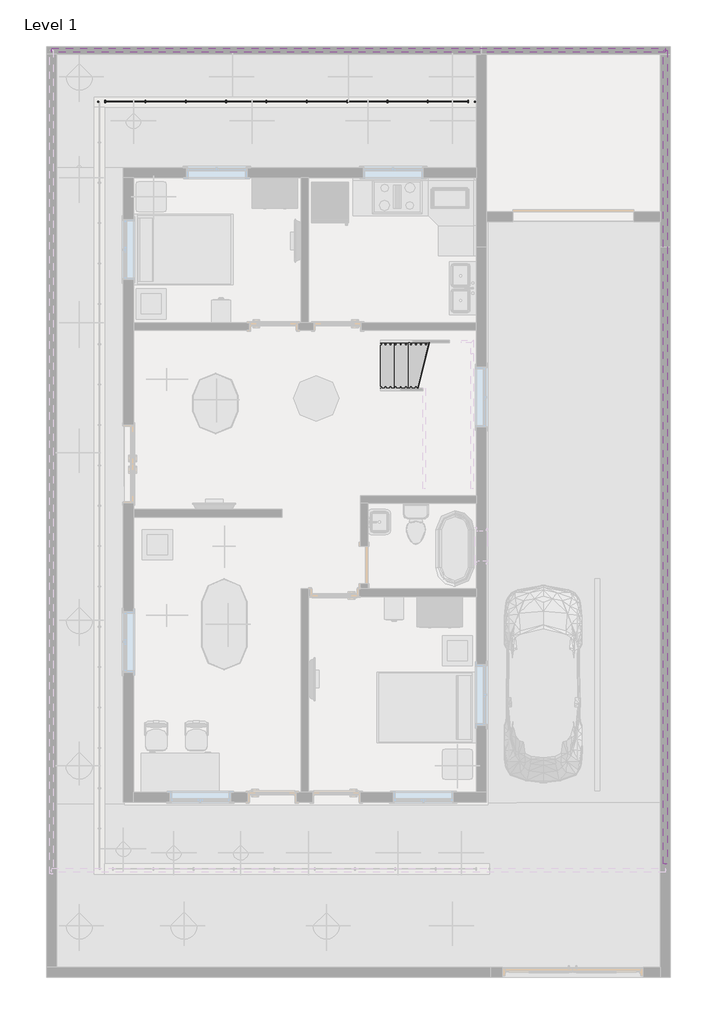
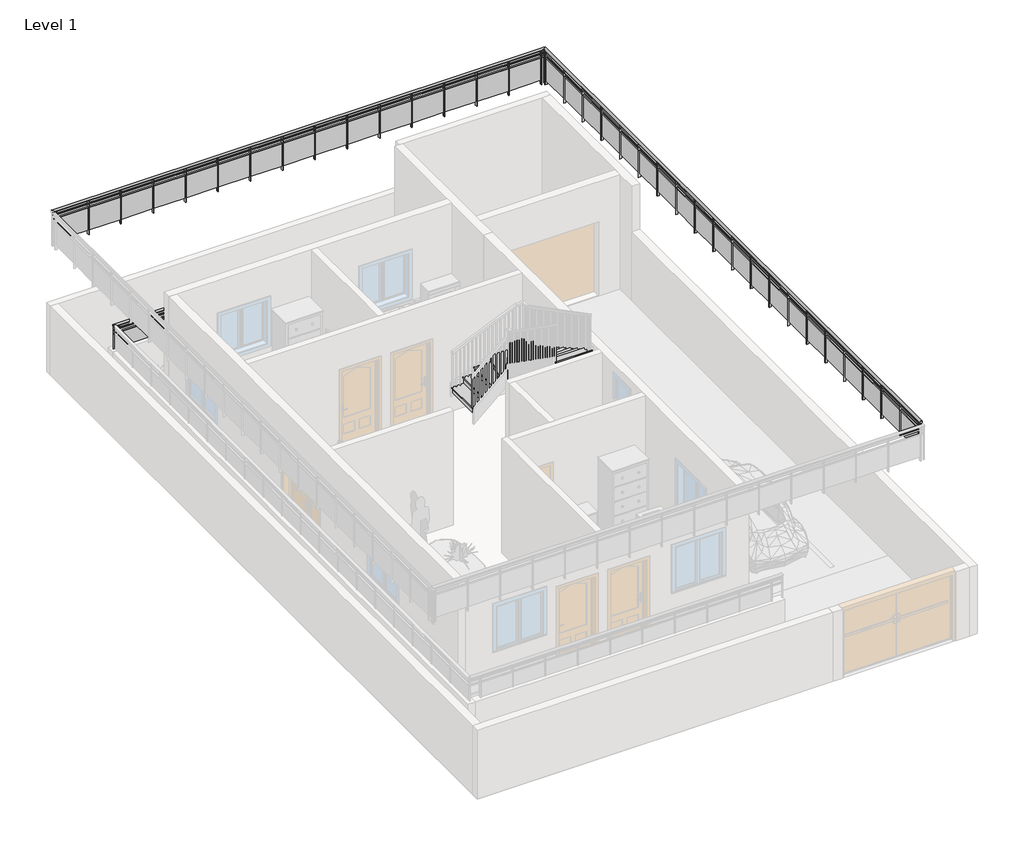
# One storey, part 4 of 5: 3 railings, 1 stair flight.
"""IFC4 building model written with IfcOpenShell, lengths in millimetres."""

from ifc_helpers import new_model, si_unit, point, frame, origin, place, context, project, spatial, polyline, ellipse_curve, trimmed, outline, extrude, transform, mapped, element, save
from ifc_brep_helpers import plane_surface, extruded_surface, advanced_brep
from components import stair_flight_29561c67

model = new_model("IFC4")

# Units and contexts
model_context = context("Model", 3, world=origin())
ifc_project = project(units=[si_unit("LENGTHUNIT", "METRE", prefix="MILLI")], contexts=[model_context])

# Site, building, storey
site = spatial("IfcSite", under=ifc_project)
building = spatial("IfcBuilding", under=site)
storey = spatial("IfcBuildingStorey", under=building, Name="Level 1", Elevation=0.0)

# Railings
placement = place(None, origin())
element("IfcRailing", 1, ObjectType="Glass Panel - Bottom Fill", at=placement, inside=storey, context=model_context, shape_type="SolidModel", body=[
    advanced_brep(
    [(-10096.3350785, 10613.9533005, 1524.0), (-10096.3350785, 10537.7533005, 1524.0), (-2501.7350785, 10613.9533005, 1524.0), (-2501.7350785, 10537.7533005, 1524.0)],
    [
        (0, 1, ellipse_curve(frame((-10096.3350785, 10575.8533005, 1524.0), z_axis=(-1.0, 0.0, 0.0), x_axis=(0.0, -1.0, 0.0)), 38.1, 28.575)),
        (1, 0, ellipse_curve(frame((-10096.3350785, 10575.8533005, 1524.0), z_axis=(-1.0, 0.0, 0.0), x_axis=(0.0, -1.0, 0.0)), 38.1, 28.575)),
        (2, 3, ellipse_curve(frame((-2501.7350785, 10575.8533005, 1524.0), z_axis=(1.0, 0.0, 0.0), x_axis=(0.0, -1.0, 0.0)), 38.1, 28.575)),
        (3, 2, ellipse_curve(frame((-2501.7350785, 10575.8533005, 1524.0), z_axis=(1.0, 0.0, 0.0), x_axis=(0.0, -1.0, 0.0)), 38.1, 28.575)),
        (0, 2),
        (3, 1),
    ],
    [
        plane_surface(frame((-10096.3350785, 10575.8533005, 1524.0), z_axis=(-1.0, 0.0, 0.0), x_axis=(0.0, 1.0, 0.0))),
        plane_surface(frame((-2501.7350785, 10575.8533005, 1524.0), z_axis=(1.0, 0.0, 0.0), x_axis=(0.0, 1.0, 0.0))),
        extruded_surface(trimmed(ellipse_curve(frame((-2501.7350785, 10575.8533005, 1524.0), z_axis=(-1.0, 0.0, 0.0), x_axis=(0.0, -1.0, 0.0)), 38.1, 28.575), [point((-2501.7350785, 10613.9533005, 1524.0))], [point((-2501.7350785, 10537.7533005, 1524.0))], True, "CARTESIAN"), (-7594.6, 0.0, 0.0), 7594.6),
        extruded_surface(trimmed(ellipse_curve(frame((-2501.7350785, 10575.8533005, 1524.0), z_axis=(-1.0, 0.0, 0.0), x_axis=(0.0, -1.0, 0.0)), 38.1, 28.575), [point((-2501.7350785, 10537.7533005, 1524.0))], [point((-2501.7350785, 10613.9533005, 1524.0))], True, "CARTESIAN"), (-7594.6, 0.0, 0.0), 7594.6),
    ],
    [
        (0, [[1, 2]]),
        (1, [[3, 4]]),
        (2, [[-1, 5, -4, 6]]),
        (3, [[-2, -6, -3, -5]]),
    ],
),
    extrude(outline(polyline([(-10096.3350785, 10563.1533005), (-10096.3350785, 10588.5533005), (-2501.7350785, 10588.5533005), (-2501.7350785, 10563.1533005), (-10096.3350785, 10563.1533005)])), frame((0.0, 0.0, 1409.7), z_axis=(0.0, 0.0, 1.0), x_axis=(1.0, 0.0, 0.0)), (0.0, 0.0, 1.0), 25.4),
    extrude(outline(polyline([(-10096.3350785, 10563.1533005), (-10096.3350785, 10588.5533005), (-2501.7350785, 10588.5533005), (-2501.7350785, 10563.1533005), (-10096.3350785, 10563.1533005)])), frame((0.0, 0.0, 1308.1), z_axis=(0.0, 0.0, 1.0), x_axis=(1.0, 0.0, 0.0)), (0.0, 0.0, 1.0), 25.4),
    extrude(outline(polyline([(-2647.7850785, 10550.4533005), (-2647.7850785, 10601.2533005), (-2635.0850785, 10601.2533005), (-2635.0850785, 10550.4533005), (-2647.7850785, 10550.4533005)])), frame((0.0, 0.0, 609.6), z_axis=(0.0, 0.0, 1.0), x_axis=(1.0, 0.0, 0.0)), (0.0, 0.0, 1.0), 885.6788223),
    extrude(outline(polyline([(-3454.2350785, 10582.3884575), (-2641.4350785, 10582.3884575), (-2641.4350785, 10576.0384575), (-3454.2350785, 10576.0384575), (-3454.2350785, 10582.3884575)])), frame((0.0, 0.0, 711.2), z_axis=(0.0, 0.0, 1.0), x_axis=(1.0, 0.0, 0.0)), (0.0, 0.0, 1.0), 596.9),
    extrude(outline(polyline([(-3460.5850785, 10550.4533005), (-3460.5850785, 10601.2533005), (-3447.8850785, 10601.2533005), (-3447.8850785, 10550.4533005), (-3460.5850785, 10550.4533005)])), frame((0.0, 0.0, 609.6), z_axis=(0.0, 0.0, 1.0), x_axis=(1.0, 0.0, 0.0)), (0.0, 0.0, 1.0), 885.6788223),
    extrude(outline(polyline([(-4267.0350785, 10582.3884575), (-3454.2350785, 10582.3884575), (-3454.2350785, 10576.0384575), (-4267.0350785, 10576.0384575), (-4267.0350785, 10582.3884575)])), frame((0.0, 0.0, 711.2), z_axis=(0.0, 0.0, 1.0), x_axis=(1.0, 0.0, 0.0)), (0.0, 0.0, 1.0), 596.9),
    extrude(outline(polyline([(-4273.3850785, 10550.4533005), (-4273.3850785, 10601.2533005), (-4260.6850785, 10601.2533005), (-4260.6850785, 10550.4533005), (-4273.3850785, 10550.4533005)])), frame((0.0, 0.0, 609.6), z_axis=(0.0, 0.0, 1.0), x_axis=(1.0, 0.0, 0.0)), (0.0, 0.0, 1.0), 885.6788223),
    extrude(outline(polyline([(-5079.8350785, 10582.3884575), (-4267.0350785, 10582.3884575), (-4267.0350785, 10576.0384575), (-5079.8350785, 10576.0384575), (-5079.8350785, 10582.3884575)])), frame((0.0, 0.0, 711.2), z_axis=(0.0, 0.0, 1.0), x_axis=(1.0, 0.0, 0.0)), (0.0, 0.0, 1.0), 596.9),
    extrude(outline(polyline([(-5086.1850785, 10550.4533005), (-5086.1850785, 10601.2533005), (-5073.4850785, 10601.2533005), (-5073.4850785, 10550.4533005), (-5086.1850785, 10550.4533005)])), frame((0.0, 0.0, 609.6), z_axis=(0.0, 0.0, 1.0), x_axis=(1.0, 0.0, 0.0)), (0.0, 0.0, 1.0), 885.6788223),
    extrude(outline(polyline([(-5892.6350785, 10582.3884575), (-5079.8350785, 10582.3884575), (-5079.8350785, 10576.0384575), (-5892.6350785, 10576.0384575), (-5892.6350785, 10582.3884575)])), frame((0.0, 0.0, 711.2), z_axis=(0.0, 0.0, 1.0), x_axis=(1.0, 0.0, 0.0)), (0.0, 0.0, 1.0), 596.9),
    extrude(outline(polyline([(-5898.9850785, 10550.4533005), (-5898.9850785, 10601.2533005), (-5886.2850785, 10601.2533005), (-5886.2850785, 10550.4533005), (-5898.9850785, 10550.4533005)])), frame((0.0, 0.0, 609.6), z_axis=(0.0, 0.0, 1.0), x_axis=(1.0, 0.0, 0.0)), (0.0, 0.0, 1.0), 885.6788223),
    extrude(outline(polyline([(-6705.4350785, 10582.3884575), (-5892.6350785, 10582.3884575), (-5892.6350785, 10576.0384575), (-6705.4350785, 10576.0384575), (-6705.4350785, 10582.3884575)])), frame((0.0, 0.0, 711.2), z_axis=(0.0, 0.0, 1.0), x_axis=(1.0, 0.0, 0.0)), (0.0, 0.0, 1.0), 596.9),
    extrude(outline(polyline([(-6711.7850785, 10550.4533005), (-6711.7850785, 10601.2533005), (-6699.0850785, 10601.2533005), (-6699.0850785, 10550.4533005), (-6711.7850785, 10550.4533005)])), frame((0.0, 0.0, 609.6), z_axis=(0.0, 0.0, 1.0), x_axis=(1.0, 0.0, 0.0)), (0.0, 0.0, 1.0), 885.6788223),
    extrude(outline(polyline([(-7518.2350785, 10582.3884575), (-6705.4350785, 10582.3884575), (-6705.4350785, 10576.0384575), (-7518.2350785, 10576.0384575), (-7518.2350785, 10582.3884575)])), frame((0.0, 0.0, 711.2), z_axis=(0.0, 0.0, 1.0), x_axis=(1.0, 0.0, 0.0)), (0.0, 0.0, 1.0), 596.9),
    extrude(outline(polyline([(-7524.5850785, 10550.4533005), (-7524.5850785, 10601.2533005), (-7511.8850785, 10601.2533005), (-7511.8850785, 10550.4533005), (-7524.5850785, 10550.4533005)])), frame((0.0, 0.0, 609.6), z_axis=(0.0, 0.0, 1.0), x_axis=(1.0, 0.0, 0.0)), (0.0, 0.0, 1.0), 885.6788223),
    extrude(outline(polyline([(-8331.0350785, 10582.3884575), (-7518.2350785, 10582.3884575), (-7518.2350785, 10576.0384575), (-8331.0350785, 10576.0384575), (-8331.0350785, 10582.3884575)])), frame((0.0, 0.0, 711.2), z_axis=(0.0, 0.0, 1.0), x_axis=(1.0, 0.0, 0.0)), (0.0, 0.0, 1.0), 596.9),
    extrude(outline(polyline([(-8337.3850785, 10550.4533005), (-8337.3850785, 10601.2533005), (-8324.6850785, 10601.2533005), (-8324.6850785, 10550.4533005), (-8337.3850785, 10550.4533005)])), frame((0.0, 0.0, 609.6), z_axis=(0.0, 0.0, 1.0), x_axis=(1.0, 0.0, 0.0)), (0.0, 0.0, 1.0), 885.6788223),
    extrude(outline(polyline([(-9143.8350785, 10582.3884575), (-8331.0350785, 10582.3884575), (-8331.0350785, 10576.0384575), (-9143.8350785, 10576.0384575), (-9143.8350785, 10582.3884575)])), frame((0.0, 0.0, 711.2), z_axis=(0.0, 0.0, 1.0), x_axis=(1.0, 0.0, 0.0)), (0.0, 0.0, 1.0), 596.9),
    extrude(outline(polyline([(-9150.1850785, 10550.4533005), (-9150.1850785, 10601.2533005), (-9137.4850785, 10601.2533005), (-9137.4850785, 10550.4533005), (-9150.1850785, 10550.4533005)])), frame((0.0, 0.0, 609.6), z_axis=(0.0, 0.0, 1.0), x_axis=(1.0, 0.0, 0.0)), (0.0, 0.0, 1.0), 885.6788223),
    extrude(outline(polyline([(-9956.6350785, 10582.3884575), (-9143.8350785, 10582.3884575), (-9143.8350785, 10576.0384575), (-9956.6350785, 10576.0384575), (-9956.6350785, 10582.3884575)])), frame((0.0, 0.0, 711.2), z_axis=(0.0, 0.0, 1.0), x_axis=(1.0, 0.0, 0.0)), (0.0, 0.0, 1.0), 596.9),
    extrude(outline(polyline([(-9962.9850785, 10550.4533005), (-9962.9850785, 10601.2533005), (-9950.2850785, 10601.2533005), (-9950.2850785, 10550.4533005), (-9962.9850785, 10550.4533005)])), frame((0.0, 0.0, 609.6), z_axis=(0.0, 0.0, 1.0), x_axis=(1.0, 0.0, 0.0)), (0.0, 0.0, 1.0), 885.6788223),
    extrude(outline(polyline([(-2514.4350785, 10566.3283005), (-2514.4350785, 10585.3783005), (-2495.3850785, 10585.3783005), (-2495.3850785, 10566.3283005), (-2514.4350785, 10566.3283005)])), frame((0.0, 0.0, 609.6), z_axis=(0.0, 0.0, 1.0), x_axis=(1.0, 0.0, 0.0)), (0.0, 0.0, 1.0), 885.6788223),
    extrude(outline(polyline([(-10102.6850785, 10566.3283005), (-10102.6850785, 10585.3783005), (-10083.6350785, 10585.3783005), (-10083.6350785, 10566.3283005), (-10102.6850785, 10566.3283005)])), frame((0.0, 0.0, 609.6), z_axis=(0.0, 0.0, 1.0), x_axis=(1.0, 0.0, 0.0)), (0.0, 0.0, 1.0), 885.6788223),
])
element("IfcRailing", 2, ObjectType="Glass Panel - Bottom Fill", at=placement, inside=storey, context=model_context, shape_type="SolidModel", body=[
    advanced_brep(
    [(-11036.1350785, 11649.0033005, 4267.2), (-11036.1350785, 11572.8033005, 4267.2), (1333.6649215, 11649.0033005, 4267.2), (1333.6649215, 11572.8033005, 4267.2)],
    [
        (0, 1, ellipse_curve(frame((-11036.1350785, 11610.9033005, 4267.2), z_axis=(-1.0, 0.0, 0.0), x_axis=(0.0, -1.0, 0.0)), 38.1, 28.575)),
        (1, 0, ellipse_curve(frame((-11036.1350785, 11610.9033005, 4267.2), z_axis=(-1.0, 0.0, 0.0), x_axis=(0.0, -1.0, 0.0)), 38.1, 28.575)),
        (2, 3, ellipse_curve(frame((1333.6649215, 11610.9033005, 4267.2), z_axis=(1.0, 0.0, 0.0), x_axis=(0.0, -1.0, 0.0)), 38.1, 28.575)),
        (3, 2, ellipse_curve(frame((1333.6649215, 11610.9033005, 4267.2), z_axis=(1.0, 0.0, 0.0), x_axis=(0.0, -1.0, 0.0)), 38.1, 28.575)),
        (0, 2),
        (3, 1),
    ],
    [
        plane_surface(frame((-11036.1350785, 11610.9033005, 4267.2), z_axis=(-1.0, 0.0, 0.0), x_axis=(0.0, 1.0, 0.0))),
        plane_surface(frame((1333.6649215, 11610.9033005, 4267.2), z_axis=(1.0, 0.0, 0.0), x_axis=(0.0, 1.0, 0.0))),
        extruded_surface(trimmed(ellipse_curve(frame((1333.6649215, 11610.9033005, 4267.2), z_axis=(-1.0, 0.0, 0.0), x_axis=(0.0, -1.0, 0.0)), 38.1, 28.575), [point((1333.6649215, 11649.0033005, 4267.2))], [point((1333.6649215, 11572.8033005, 4267.2))], True, "CARTESIAN"), (-12369.8, 0.0, 0.0), 12369.8),
        extruded_surface(trimmed(ellipse_curve(frame((1333.6649215, 11610.9033005, 4267.2), z_axis=(-1.0, 0.0, 0.0), x_axis=(0.0, -1.0, 0.0)), 38.1, 28.575), [point((1333.6649215, 11572.8033005, 4267.2))], [point((1333.6649215, 11649.0033005, 4267.2))], True, "CARTESIAN"), (-12369.8, 0.0, 0.0), 12369.8),
    ],
    [
        (0, [[1, 2]]),
        (1, [[3, 4]]),
        (2, [[-1, 5, -4, 6]]),
        (3, [[-2, -6, -3, -5]]),
    ],
),
    extrude(outline(polyline([(-11036.1350785, 11598.2033005), (-11036.1350785, 11623.6033005), (1333.6649215, 11623.6033005), (1333.6649215, 11598.2033005), (-11036.1350785, 11598.2033005)])), frame((0.0, 0.0, 4152.9), z_axis=(0.0, 0.0, 1.0), x_axis=(1.0, 0.0, 0.0)), (0.0, 0.0, 1.0), 25.4),
    extrude(outline(polyline([(-11036.1350785, 11598.2033005), (-11036.1350785, 11623.6033005), (1333.6649215, 11623.6033005), (1333.6649215, 11598.2033005), (-11036.1350785, 11598.2033005)])), frame((0.0, 0.0, 4051.3), z_axis=(0.0, 0.0, 1.0), x_axis=(1.0, 0.0, 0.0)), (0.0, 0.0, 1.0), 25.4),
    extrude(outline(polyline([(1238.4149215, 11585.5033005), (1238.4149215, 11636.3033005), (1251.1149215, 11636.3033005), (1251.1149215, 11585.5033005), (1238.4149215, 11585.5033005)])), frame((0.0, 0.0, 3352.8), z_axis=(0.0, 0.0, 1.0), x_axis=(1.0, 0.0, 0.0)), (0.0, 0.0, 1.0), 885.6788223),
    extrude(outline(polyline([(431.9649215, 11617.4384575), (1244.7649215, 11617.4384575), (1244.7649215, 11611.0884575), (431.9649215, 11611.0884575), (431.9649215, 11617.4384575)])), frame((0.0, 0.0, 3454.4), z_axis=(0.0, 0.0, 1.0), x_axis=(1.0, 0.0, 0.0)), (0.0, 0.0, 1.0), 596.9),
    extrude(outline(polyline([(425.6149215, 11585.5033005), (425.6149215, 11636.3033005), (438.3149215, 11636.3033005), (438.3149215, 11585.5033005), (425.6149215, 11585.5033005)])), frame((0.0, 0.0, 3352.8), z_axis=(0.0, 0.0, 1.0), x_axis=(1.0, 0.0, 0.0)), (0.0, 0.0, 1.0), 885.6788223),
    extrude(outline(polyline([(-380.8350785, 11617.4384575), (431.9649215, 11617.4384575), (431.9649215, 11611.0884575), (-380.8350785, 11611.0884575), (-380.8350785, 11617.4384575)])), frame((0.0, 0.0, 3454.4), z_axis=(0.0, 0.0, 1.0), x_axis=(1.0, 0.0, 0.0)), (0.0, 0.0, 1.0), 596.9),
    extrude(outline(polyline([(-387.1850785, 11585.5033005), (-387.1850785, 11636.3033005), (-374.4850785, 11636.3033005), (-374.4850785, 11585.5033005), (-387.1850785, 11585.5033005)])), frame((0.0, 0.0, 3352.8), z_axis=(0.0, 0.0, 1.0), x_axis=(1.0, 0.0, 0.0)), (0.0, 0.0, 1.0), 885.6788223),
    extrude(outline(polyline([(-1193.6350785, 11617.4384575), (-380.8350785, 11617.4384575), (-380.8350785, 11611.0884575), (-1193.6350785, 11611.0884575), (-1193.6350785, 11617.4384575)])), frame((0.0, 0.0, 3454.4), z_axis=(0.0, 0.0, 1.0), x_axis=(1.0, 0.0, 0.0)), (0.0, 0.0, 1.0), 596.9),
    extrude(outline(polyline([(-1199.9850785, 11585.5033005), (-1199.9850785, 11636.3033005), (-1187.2850785, 11636.3033005), (-1187.2850785, 11585.5033005), (-1199.9850785, 11585.5033005)])), frame((0.0, 0.0, 3352.8), z_axis=(0.0, 0.0, 1.0), x_axis=(1.0, 0.0, 0.0)), (0.0, 0.0, 1.0), 885.6788223),
    extrude(outline(polyline([(-2006.4350785, 11617.4384575), (-1193.6350785, 11617.4384575), (-1193.6350785, 11611.0884575), (-2006.4350785, 11611.0884575), (-2006.4350785, 11617.4384575)])), frame((0.0, 0.0, 3454.4), z_axis=(0.0, 0.0, 1.0), x_axis=(1.0, 0.0, 0.0)), (0.0, 0.0, 1.0), 596.9),
    extrude(outline(polyline([(-2012.7850785, 11585.5033005), (-2012.7850785, 11636.3033005), (-2000.0850785, 11636.3033005), (-2000.0850785, 11585.5033005), (-2012.7850785, 11585.5033005)])), frame((0.0, 0.0, 3352.8), z_axis=(0.0, 0.0, 1.0), x_axis=(1.0, 0.0, 0.0)), (0.0, 0.0, 1.0), 885.6788223),
    extrude(outline(polyline([(-2819.2350785, 11617.4384575), (-2006.4350785, 11617.4384575), (-2006.4350785, 11611.0884575), (-2819.2350785, 11611.0884575), (-2819.2350785, 11617.4384575)])), frame((0.0, 0.0, 3454.4), z_axis=(0.0, 0.0, 1.0), x_axis=(1.0, 0.0, 0.0)), (0.0, 0.0, 1.0), 596.9),
    extrude(outline(polyline([(-2825.5850785, 11585.5033005), (-2825.5850785, 11636.3033005), (-2812.8850785, 11636.3033005), (-2812.8850785, 11585.5033005), (-2825.5850785, 11585.5033005)])), frame((0.0, 0.0, 3352.8), z_axis=(0.0, 0.0, 1.0), x_axis=(1.0, 0.0, 0.0)), (0.0, 0.0, 1.0), 885.6788223),
    extrude(outline(polyline([(-3632.0350785, 11617.4384575), (-2819.2350785, 11617.4384575), (-2819.2350785, 11611.0884575), (-3632.0350785, 11611.0884575), (-3632.0350785, 11617.4384575)])), frame((0.0, 0.0, 3454.4), z_axis=(0.0, 0.0, 1.0), x_axis=(1.0, 0.0, 0.0)), (0.0, 0.0, 1.0), 596.9),
    extrude(outline(polyline([(-3638.3850785, 11585.5033005), (-3638.3850785, 11636.3033005), (-3625.6850785, 11636.3033005), (-3625.6850785, 11585.5033005), (-3638.3850785, 11585.5033005)])), frame((0.0, 0.0, 3352.8), z_axis=(0.0, 0.0, 1.0), x_axis=(1.0, 0.0, 0.0)), (0.0, 0.0, 1.0), 885.6788223),
    extrude(outline(polyline([(-4444.8350785, 11617.4384575), (-3632.0350785, 11617.4384575), (-3632.0350785, 11611.0884575), (-4444.8350785, 11611.0884575), (-4444.8350785, 11617.4384575)])), frame((0.0, 0.0, 3454.4), z_axis=(0.0, 0.0, 1.0), x_axis=(1.0, 0.0, 0.0)), (0.0, 0.0, 1.0), 596.9),
    extrude(outline(polyline([(-4451.1850785, 11585.5033005), (-4451.1850785, 11636.3033005), (-4438.4850785, 11636.3033005), (-4438.4850785, 11585.5033005), (-4451.1850785, 11585.5033005)])), frame((0.0, 0.0, 3352.8), z_axis=(0.0, 0.0, 1.0), x_axis=(1.0, 0.0, 0.0)), (0.0, 0.0, 1.0), 885.6788223),
    extrude(outline(polyline([(-5257.6350785, 11617.4384575), (-4444.8350785, 11617.4384575), (-4444.8350785, 11611.0884575), (-5257.6350785, 11611.0884575), (-5257.6350785, 11617.4384575)])), frame((0.0, 0.0, 3454.4), z_axis=(0.0, 0.0, 1.0), x_axis=(1.0, 0.0, 0.0)), (0.0, 0.0, 1.0), 596.9),
    extrude(outline(polyline([(-5263.9850785, 11585.5033005), (-5263.9850785, 11636.3033005), (-5251.2850785, 11636.3033005), (-5251.2850785, 11585.5033005), (-5263.9850785, 11585.5033005)])), frame((0.0, 0.0, 3352.8), z_axis=(0.0, 0.0, 1.0), x_axis=(1.0, 0.0, 0.0)), (0.0, 0.0, 1.0), 885.6788223),
    extrude(outline(polyline([(-6070.4350785, 11617.4384575), (-5257.6350785, 11617.4384575), (-5257.6350785, 11611.0884575), (-6070.4350785, 11611.0884575), (-6070.4350785, 11617.4384575)])), frame((0.0, 0.0, 3454.4), z_axis=(0.0, 0.0, 1.0), x_axis=(1.0, 0.0, 0.0)), (0.0, 0.0, 1.0), 596.9),
    extrude(outline(polyline([(-6076.7850785, 11585.5033005), (-6076.7850785, 11636.3033005), (-6064.0850785, 11636.3033005), (-6064.0850785, 11585.5033005), (-6076.7850785, 11585.5033005)])), frame((0.0, 0.0, 3352.8), z_axis=(0.0, 0.0, 1.0), x_axis=(1.0, 0.0, 0.0)), (0.0, 0.0, 1.0), 885.6788223),
    extrude(outline(polyline([(-6883.2350785, 11617.4384575), (-6070.4350785, 11617.4384575), (-6070.4350785, 11611.0884575), (-6883.2350785, 11611.0884575), (-6883.2350785, 11617.4384575)])), frame((0.0, 0.0, 3454.4), z_axis=(0.0, 0.0, 1.0), x_axis=(1.0, 0.0, 0.0)), (0.0, 0.0, 1.0), 596.9),
    extrude(outline(polyline([(-6889.5850785, 11585.5033005), (-6889.5850785, 11636.3033005), (-6876.8850785, 11636.3033005), (-6876.8850785, 11585.5033005), (-6889.5850785, 11585.5033005)])), frame((0.0, 0.0, 3352.8), z_axis=(0.0, 0.0, 1.0), x_axis=(1.0, 0.0, 0.0)), (0.0, 0.0, 1.0), 885.6788223),
    extrude(outline(polyline([(-7696.0350785, 11617.4384575), (-6883.2350785, 11617.4384575), (-6883.2350785, 11611.0884575), (-7696.0350785, 11611.0884575), (-7696.0350785, 11617.4384575)])), frame((0.0, 0.0, 3454.4), z_axis=(0.0, 0.0, 1.0), x_axis=(1.0, 0.0, 0.0)), (0.0, 0.0, 1.0), 596.9),
    extrude(outline(polyline([(-7702.3850785, 11585.5033005), (-7702.3850785, 11636.3033005), (-7689.6850785, 11636.3033005), (-7689.6850785, 11585.5033005), (-7702.3850785, 11585.5033005)])), frame((0.0, 0.0, 3352.8), z_axis=(0.0, 0.0, 1.0), x_axis=(1.0, 0.0, 0.0)), (0.0, 0.0, 1.0), 885.6788223),
    extrude(outline(polyline([(-8508.8350785, 11617.4384575), (-7696.0350785, 11617.4384575), (-7696.0350785, 11611.0884575), (-8508.8350785, 11611.0884575), (-8508.8350785, 11617.4384575)])), frame((0.0, 0.0, 3454.4), z_axis=(0.0, 0.0, 1.0), x_axis=(1.0, 0.0, 0.0)), (0.0, 0.0, 1.0), 596.9),
    extrude(outline(polyline([(-8515.1850785, 11585.5033005), (-8515.1850785, 11636.3033005), (-8502.4850785, 11636.3033005), (-8502.4850785, 11585.5033005), (-8515.1850785, 11585.5033005)])), frame((0.0, 0.0, 3352.8), z_axis=(0.0, 0.0, 1.0), x_axis=(1.0, 0.0, 0.0)), (0.0, 0.0, 1.0), 885.6788223),
    extrude(outline(polyline([(-9321.6350785, 11617.4384575), (-8508.8350785, 11617.4384575), (-8508.8350785, 11611.0884575), (-9321.6350785, 11611.0884575), (-9321.6350785, 11617.4384575)])), frame((0.0, 0.0, 3454.4), z_axis=(0.0, 0.0, 1.0), x_axis=(1.0, 0.0, 0.0)), (0.0, 0.0, 1.0), 596.9),
    extrude(outline(polyline([(-9327.9850785, 11585.5033005), (-9327.9850785, 11636.3033005), (-9315.2850785, 11636.3033005), (-9315.2850785, 11585.5033005), (-9327.9850785, 11585.5033005)])), frame((0.0, 0.0, 3352.8), z_axis=(0.0, 0.0, 1.0), x_axis=(1.0, 0.0, 0.0)), (0.0, 0.0, 1.0), 885.6788223),
    extrude(outline(polyline([(-10134.4350785, 11617.4384575), (-9321.6350785, 11617.4384575), (-9321.6350785, 11611.0884575), (-10134.4350785, 11611.0884575), (-10134.4350785, 11617.4384575)])), frame((0.0, 0.0, 3454.4), z_axis=(0.0, 0.0, 1.0), x_axis=(1.0, 0.0, 0.0)), (0.0, 0.0, 1.0), 596.9),
    extrude(outline(polyline([(-10140.7850785, 11585.5033005), (-10140.7850785, 11636.3033005), (-10128.0850785, 11636.3033005), (-10128.0850785, 11585.5033005), (-10140.7850785, 11585.5033005)])), frame((0.0, 0.0, 3352.8), z_axis=(0.0, 0.0, 1.0), x_axis=(1.0, 0.0, 0.0)), (0.0, 0.0, 1.0), 885.6788223),
    extrude(outline(polyline([(-10947.2350785, 11617.4384575), (-10134.4350785, 11617.4384575), (-10134.4350785, 11611.0884575), (-10947.2350785, 11611.0884575), (-10947.2350785, 11617.4384575)])), frame((0.0, 0.0, 3454.4), z_axis=(0.0, 0.0, 1.0), x_axis=(1.0, 0.0, 0.0)), (0.0, 0.0, 1.0), 596.9),
    extrude(outline(polyline([(-10953.5850785, 11585.5033005), (-10953.5850785, 11636.3033005), (-10940.8850785, 11636.3033005), (-10940.8850785, 11585.5033005), (-10953.5850785, 11585.5033005)])), frame((0.0, 0.0, 3352.8), z_axis=(0.0, 0.0, 1.0), x_axis=(1.0, 0.0, 0.0)), (0.0, 0.0, 1.0), 885.6788223),
    extrude(outline(polyline([(1320.9649215, 11601.3783005), (1320.9649215, 11620.4283005), (1340.0149215, 11620.4283005), (1340.0149215, 11601.3783005), (1320.9649215, 11601.3783005)])), frame((0.0, 0.0, 3352.8), z_axis=(0.0, 0.0, 1.0), x_axis=(1.0, 0.0, 0.0)), (0.0, 0.0, 1.0), 885.6788223),
    extrude(outline(polyline([(-11042.4850785, 11601.3783005), (-11042.4850785, 11620.4283005), (-11023.4350785, 11620.4283005), (-11023.4350785, 11601.3783005), (-11042.4850785, 11601.3783005)])), frame((0.0, 0.0, 3352.8), z_axis=(0.0, 0.0, 1.0), x_axis=(1.0, 0.0, 0.0)), (0.0, 0.0, 1.0), 885.6788223),
])
element("IfcRailing", 3, ObjectType="Glass Panel - Bottom Fill", at=placement, inside=storey, context=model_context, shape_type="SolidModel", body=[
    advanced_brep(
    [(1371.7649215, 11610.9033005, 4267.2), (1295.5649215, 11610.9033005, 4267.2), (1371.7649215, -4772.0966995, 4267.2), (1295.5649215, -4772.0966995, 4267.2)],
    [
        (0, 1, ellipse_curve(frame((1333.6649215, 11610.9033005, 4267.2), z_axis=(0.0, 1.0, 0.0), x_axis=(-1.0, 0.0, 0.0)), 38.1, 28.575)),
        (1, 0, ellipse_curve(frame((1333.6649215, 11610.9033005, 4267.2), z_axis=(0.0, 1.0, 0.0), x_axis=(-1.0, 0.0, 0.0)), 38.1, 28.575)),
        (2, 3, ellipse_curve(frame((1333.6649215, -4772.0966995, 4267.2), z_axis=(0.0, -1.0, 0.0), x_axis=(-1.0, 0.0, 0.0)), 38.1, 28.575)),
        (3, 2, ellipse_curve(frame((1333.6649215, -4772.0966995, 4267.2), z_axis=(0.0, -1.0, 0.0), x_axis=(-1.0, 0.0, 0.0)), 38.1, 28.575)),
        (0, 2),
        (3, 1),
    ],
    [
        plane_surface(frame((1333.6649215, 11610.9033005, 4267.2), z_axis=(0.0, 1.0, 0.0), x_axis=(0.0, 0.0, -1.0))),
        plane_surface(frame((1333.6649215, -4772.0966995, 4267.2), z_axis=(0.0, -1.0, 0.0), x_axis=(0.0, 0.0, -1.0))),
        extruded_surface(trimmed(ellipse_curve(frame((1333.6649215, -4772.0966995, 4267.2), z_axis=(0.0, 1.0, 0.0), x_axis=(-1.0, 0.0, 0.0)), 38.1, 28.575), [point((1371.7649215, -4772.0966995, 4267.2))], [point((1295.5649215, -4772.0966995, 4267.2))], True, "CARTESIAN"), (0.0, 16383.0, 0.0), 16383.0),
        extruded_surface(trimmed(ellipse_curve(frame((1333.6649215, -4772.0966995, 4267.2), z_axis=(0.0, 1.0, 0.0), x_axis=(-1.0, 0.0, 0.0)), 38.1, 28.575), [point((1295.5649215, -4772.0966995, 4267.2))], [point((1371.7649215, -4772.0966995, 4267.2))], True, "CARTESIAN"), (0.0, 16383.0, 0.0), 16383.0),
    ],
    [
        (0, [[1, 2]]),
        (1, [[3, 4]]),
        (2, [[-1, 5, -4, 6]]),
        (3, [[-2, -6, -3, -5]]),
    ],
),
    extrude(outline(polyline([(1320.9649215, 11610.9033005), (1346.3649215, 11610.9033005), (1346.3649215, -4772.0966995), (1320.9649215, -4772.0966995), (1320.9649215, 11610.9033005)])), frame((0.0, 0.0, 4152.9), z_axis=(0.0, 0.0, 1.0), x_axis=(1.0, 0.0, 0.0)), (0.0, 0.0, 1.0), 25.4),
    extrude(outline(polyline([(1320.9649215, 11610.9033005), (1346.3649215, 11610.9033005), (1346.3649215, -4772.0966995), (1320.9649215, -4772.0966995), (1320.9649215, 11610.9033005)])), frame((0.0, 0.0, 4051.3), z_axis=(0.0, 0.0, 1.0), x_axis=(1.0, 0.0, 0.0)), (0.0, 0.0, 1.0), 25.4),
    extrude(outline(polyline([(1308.2649215, -4702.2466995), (1359.0649215, -4702.2466995), (1359.0649215, -4714.9466995), (1308.2649215, -4714.9466995), (1308.2649215, -4702.2466995)])), frame((0.0, 0.0, 3352.8), z_axis=(0.0, 0.0, 1.0), x_axis=(1.0, 0.0, 0.0)), (0.0, 0.0, 1.0), 885.6788223),
    extrude(outline(polyline([(1340.2000785, -3895.7966995), (1340.2000785, -4708.5966995), (1333.8500785, -4708.5966995), (1333.8500785, -3895.7966995), (1340.2000785, -3895.7966995)])), frame((0.0, 0.0, 3454.4), z_axis=(0.0, 0.0, 1.0), x_axis=(1.0, 0.0, 0.0)), (0.0, 0.0, 1.0), 596.9),
    extrude(outline(polyline([(1308.2649215, -3889.4466995), (1359.0649215, -3889.4466995), (1359.0649215, -3902.1466995), (1308.2649215, -3902.1466995), (1308.2649215, -3889.4466995)])), frame((0.0, 0.0, 3352.8), z_axis=(0.0, 0.0, 1.0), x_axis=(1.0, 0.0, 0.0)), (0.0, 0.0, 1.0), 885.6788223),
    extrude(outline(polyline([(1340.2000785, -3082.9966995), (1340.2000785, -3895.7966995), (1333.8500785, -3895.7966995), (1333.8500785, -3082.9966995), (1340.2000785, -3082.9966995)])), frame((0.0, 0.0, 3454.4), z_axis=(0.0, 0.0, 1.0), x_axis=(1.0, 0.0, 0.0)), (0.0, 0.0, 1.0), 596.9),
    extrude(outline(polyline([(1308.2649215, -3076.6466995), (1359.0649215, -3076.6466995), (1359.0649215, -3089.3466995), (1308.2649215, -3089.3466995), (1308.2649215, -3076.6466995)])), frame((0.0, 0.0, 3352.8), z_axis=(0.0, 0.0, 1.0), x_axis=(1.0, 0.0, 0.0)), (0.0, 0.0, 1.0), 885.6788223),
    extrude(outline(polyline([(1340.2000785, -2270.1966995), (1340.2000785, -3082.9966995), (1333.8500785, -3082.9966995), (1333.8500785, -2270.1966995), (1340.2000785, -2270.1966995)])), frame((0.0, 0.0, 3454.4), z_axis=(0.0, 0.0, 1.0), x_axis=(1.0, 0.0, 0.0)), (0.0, 0.0, 1.0), 596.9),
    extrude(outline(polyline([(1308.2649215, -2263.8466995), (1359.0649215, -2263.8466995), (1359.0649215, -2276.5466995), (1308.2649215, -2276.5466995), (1308.2649215, -2263.8466995)])), frame((0.0, 0.0, 3352.8), z_axis=(0.0, 0.0, 1.0), x_axis=(1.0, 0.0, 0.0)), (0.0, 0.0, 1.0), 885.6788223),
    extrude(outline(polyline([(1340.2000785, -1457.3966995), (1340.2000785, -2270.1966995), (1333.8500785, -2270.1966995), (1333.8500785, -1457.3966995), (1340.2000785, -1457.3966995)])), frame((0.0, 0.0, 3454.4), z_axis=(0.0, 0.0, 1.0), x_axis=(1.0, 0.0, 0.0)), (0.0, 0.0, 1.0), 596.9),
    extrude(outline(polyline([(1308.2649215, -1451.0466995), (1359.0649215, -1451.0466995), (1359.0649215, -1463.7466995), (1308.2649215, -1463.7466995), (1308.2649215, -1451.0466995)])), frame((0.0, 0.0, 3352.8), z_axis=(0.0, 0.0, 1.0), x_axis=(1.0, 0.0, 0.0)), (0.0, 0.0, 1.0), 885.6788223),
    extrude(outline(polyline([(1340.2000785, -644.5966995), (1340.2000785, -1457.3966995), (1333.8500785, -1457.3966995), (1333.8500785, -644.5966995), (1340.2000785, -644.5966995)])), frame((0.0, 0.0, 3454.4), z_axis=(0.0, 0.0, 1.0), x_axis=(1.0, 0.0, 0.0)), (0.0, 0.0, 1.0), 596.9),
    extrude(outline(polyline([(1308.2649215, -638.2466995), (1359.0649215, -638.2466995), (1359.0649215, -650.9466995), (1308.2649215, -650.9466995), (1308.2649215, -638.2466995)])), frame((0.0, 0.0, 3352.8), z_axis=(0.0, 0.0, 1.0), x_axis=(1.0, 0.0, 0.0)), (0.0, 0.0, 1.0), 885.6788223),
    extrude(outline(polyline([(1340.2000785, 168.2033005), (1340.2000785, -644.5966995), (1333.8500785, -644.5966995), (1333.8500785, 168.2033005), (1340.2000785, 168.2033005)])), frame((0.0, 0.0, 3454.4), z_axis=(0.0, 0.0, 1.0), x_axis=(1.0, 0.0, 0.0)), (0.0, 0.0, 1.0), 596.9),
    extrude(outline(polyline([(1308.2649215, 174.5533005), (1359.0649215, 174.5533005), (1359.0649215, 161.8533005), (1308.2649215, 161.8533005), (1308.2649215, 174.5533005)])), frame((0.0, 0.0, 3352.8), z_axis=(0.0, 0.0, 1.0), x_axis=(1.0, 0.0, 0.0)), (0.0, 0.0, 1.0), 885.6788223),
    extrude(outline(polyline([(1340.2000785, 981.0033005), (1340.2000785, 168.2033005), (1333.8500785, 168.2033005), (1333.8500785, 981.0033005), (1340.2000785, 981.0033005)])), frame((0.0, 0.0, 3454.4), z_axis=(0.0, 0.0, 1.0), x_axis=(1.0, 0.0, 0.0)), (0.0, 0.0, 1.0), 596.9),
    extrude(outline(polyline([(1308.2649215, 987.3533005), (1359.0649215, 987.3533005), (1359.0649215, 974.6533005), (1308.2649215, 974.6533005), (1308.2649215, 987.3533005)])), frame((0.0, 0.0, 3352.8), z_axis=(0.0, 0.0, 1.0), x_axis=(1.0, 0.0, 0.0)), (0.0, 0.0, 1.0), 885.6788223),
    extrude(outline(polyline([(1340.2000785, 1793.8033005), (1340.2000785, 981.0033005), (1333.8500785, 981.0033005), (1333.8500785, 1793.8033005), (1340.2000785, 1793.8033005)])), frame((0.0, 0.0, 3454.4), z_axis=(0.0, 0.0, 1.0), x_axis=(1.0, 0.0, 0.0)), (0.0, 0.0, 1.0), 596.9),
    extrude(outline(polyline([(1308.2649215, 1800.1533005), (1359.0649215, 1800.1533005), (1359.0649215, 1787.4533005), (1308.2649215, 1787.4533005), (1308.2649215, 1800.1533005)])), frame((0.0, 0.0, 3352.8), z_axis=(0.0, 0.0, 1.0), x_axis=(1.0, 0.0, 0.0)), (0.0, 0.0, 1.0), 885.6788223),
    extrude(outline(polyline([(1340.2000785, 2606.6033005), (1340.2000785, 1793.8033005), (1333.8500785, 1793.8033005), (1333.8500785, 2606.6033005), (1340.2000785, 2606.6033005)])), frame((0.0, 0.0, 3454.4), z_axis=(0.0, 0.0, 1.0), x_axis=(1.0, 0.0, 0.0)), (0.0, 0.0, 1.0), 596.9),
    extrude(outline(polyline([(1308.2649215, 2612.9533005), (1359.0649215, 2612.9533005), (1359.0649215, 2600.2533005), (1308.2649215, 2600.2533005), (1308.2649215, 2612.9533005)])), frame((0.0, 0.0, 3352.8), z_axis=(0.0, 0.0, 1.0), x_axis=(1.0, 0.0, 0.0)), (0.0, 0.0, 1.0), 885.6788223),
    extrude(outline(polyline([(1340.2000785, 3419.4033005), (1340.2000785, 2606.6033005), (1333.8500785, 2606.6033005), (1333.8500785, 3419.4033005), (1340.2000785, 3419.4033005)])), frame((0.0, 0.0, 3454.4), z_axis=(0.0, 0.0, 1.0), x_axis=(1.0, 0.0, 0.0)), (0.0, 0.0, 1.0), 596.9),
    extrude(outline(polyline([(1308.2649215, 3425.7533005), (1359.0649215, 3425.7533005), (1359.0649215, 3413.0533005), (1308.2649215, 3413.0533005), (1308.2649215, 3425.7533005)])), frame((0.0, 0.0, 3352.8), z_axis=(0.0, 0.0, 1.0), x_axis=(1.0, 0.0, 0.0)), (0.0, 0.0, 1.0), 885.6788223),
    extrude(outline(polyline([(1340.2000785, 4232.2033005), (1340.2000785, 3419.4033005), (1333.8500785, 3419.4033005), (1333.8500785, 4232.2033005), (1340.2000785, 4232.2033005)])), frame((0.0, 0.0, 3454.4), z_axis=(0.0, 0.0, 1.0), x_axis=(1.0, 0.0, 0.0)), (0.0, 0.0, 1.0), 596.9),
    extrude(outline(polyline([(1308.2649215, 4238.5533005), (1359.0649215, 4238.5533005), (1359.0649215, 4225.8533005), (1308.2649215, 4225.8533005), (1308.2649215, 4238.5533005)])), frame((0.0, 0.0, 3352.8), z_axis=(0.0, 0.0, 1.0), x_axis=(1.0, 0.0, 0.0)), (0.0, 0.0, 1.0), 885.6788223),
    extrude(outline(polyline([(1340.2000785, 5045.0033005), (1340.2000785, 4232.2033005), (1333.8500785, 4232.2033005), (1333.8500785, 5045.0033005), (1340.2000785, 5045.0033005)])), frame((0.0, 0.0, 3454.4), z_axis=(0.0, 0.0, 1.0), x_axis=(1.0, 0.0, 0.0)), (0.0, 0.0, 1.0), 596.9),
    extrude(outline(polyline([(1308.2649215, 5051.3533005), (1359.0649215, 5051.3533005), (1359.0649215, 5038.6533005), (1308.2649215, 5038.6533005), (1308.2649215, 5051.3533005)])), frame((0.0, 0.0, 3352.8), z_axis=(0.0, 0.0, 1.0), x_axis=(1.0, 0.0, 0.0)), (0.0, 0.0, 1.0), 885.6788223),
    extrude(outline(polyline([(1340.2000785, 5857.8033005), (1340.2000785, 5045.0033005), (1333.8500785, 5045.0033005), (1333.8500785, 5857.8033005), (1340.2000785, 5857.8033005)])), frame((0.0, 0.0, 3454.4), z_axis=(0.0, 0.0, 1.0), x_axis=(1.0, 0.0, 0.0)), (0.0, 0.0, 1.0), 596.9),
    extrude(outline(polyline([(1308.2649215, 5864.1533005), (1359.0649215, 5864.1533005), (1359.0649215, 5851.4533005), (1308.2649215, 5851.4533005), (1308.2649215, 5864.1533005)])), frame((0.0, 0.0, 3352.8), z_axis=(0.0, 0.0, 1.0), x_axis=(1.0, 0.0, 0.0)), (0.0, 0.0, 1.0), 885.6788223),
    extrude(outline(polyline([(1340.2000785, 6670.6033005), (1340.2000785, 5857.8033005), (1333.8500785, 5857.8033005), (1333.8500785, 6670.6033005), (1340.2000785, 6670.6033005)])), frame((0.0, 0.0, 3454.4), z_axis=(0.0, 0.0, 1.0), x_axis=(1.0, 0.0, 0.0)), (0.0, 0.0, 1.0), 596.9),
    extrude(outline(polyline([(1308.2649215, 6676.9533005), (1359.0649215, 6676.9533005), (1359.0649215, 6664.2533005), (1308.2649215, 6664.2533005), (1308.2649215, 6676.9533005)])), frame((0.0, 0.0, 3352.8), z_axis=(0.0, 0.0, 1.0), x_axis=(1.0, 0.0, 0.0)), (0.0, 0.0, 1.0), 885.6788223),
    extrude(outline(polyline([(1340.2000785, 7483.4033005), (1340.2000785, 6670.6033005), (1333.8500785, 6670.6033005), (1333.8500785, 7483.4033005), (1340.2000785, 7483.4033005)])), frame((0.0, 0.0, 3454.4), z_axis=(0.0, 0.0, 1.0), x_axis=(1.0, 0.0, 0.0)), (0.0, 0.0, 1.0), 596.9),
    extrude(outline(polyline([(1308.2649215, 7489.7533005), (1359.0649215, 7489.7533005), (1359.0649215, 7477.0533005), (1308.2649215, 7477.0533005), (1308.2649215, 7489.7533005)])), frame((0.0, 0.0, 3352.8), z_axis=(0.0, 0.0, 1.0), x_axis=(1.0, 0.0, 0.0)), (0.0, 0.0, 1.0), 885.6788223),
    extrude(outline(polyline([(1340.2000785, 8296.2033005), (1340.2000785, 7483.4033005), (1333.8500785, 7483.4033005), (1333.8500785, 8296.2033005), (1340.2000785, 8296.2033005)])), frame((0.0, 0.0, 3454.4), z_axis=(0.0, 0.0, 1.0), x_axis=(1.0, 0.0, 0.0)), (0.0, 0.0, 1.0), 596.9),
    extrude(outline(polyline([(1308.2649215, 8302.5533005), (1359.0649215, 8302.5533005), (1359.0649215, 8289.8533005), (1308.2649215, 8289.8533005), (1308.2649215, 8302.5533005)])), frame((0.0, 0.0, 3352.8), z_axis=(0.0, 0.0, 1.0), x_axis=(1.0, 0.0, 0.0)), (0.0, 0.0, 1.0), 885.6788223),
    extrude(outline(polyline([(1340.2000785, 9109.0033005), (1340.2000785, 8296.2033005), (1333.8500785, 8296.2033005), (1333.8500785, 9109.0033005), (1340.2000785, 9109.0033005)])), frame((0.0, 0.0, 3454.4), z_axis=(0.0, 0.0, 1.0), x_axis=(1.0, 0.0, 0.0)), (0.0, 0.0, 1.0), 596.9),
    extrude(outline(polyline([(1308.2649215, 9115.3533005), (1359.0649215, 9115.3533005), (1359.0649215, 9102.6533005), (1308.2649215, 9102.6533005), (1308.2649215, 9115.3533005)])), frame((0.0, 0.0, 3352.8), z_axis=(0.0, 0.0, 1.0), x_axis=(1.0, 0.0, 0.0)), (0.0, 0.0, 1.0), 885.6788223),
    extrude(outline(polyline([(1340.2000785, 9921.8033005), (1340.2000785, 9109.0033005), (1333.8500785, 9109.0033005), (1333.8500785, 9921.8033005), (1340.2000785, 9921.8033005)])), frame((0.0, 0.0, 3454.4), z_axis=(0.0, 0.0, 1.0), x_axis=(1.0, 0.0, 0.0)), (0.0, 0.0, 1.0), 596.9),
    extrude(outline(polyline([(1308.2649215, 9928.1533005), (1359.0649215, 9928.1533005), (1359.0649215, 9915.4533005), (1308.2649215, 9915.4533005), (1308.2649215, 9928.1533005)])), frame((0.0, 0.0, 3352.8), z_axis=(0.0, 0.0, 1.0), x_axis=(1.0, 0.0, 0.0)), (0.0, 0.0, 1.0), 885.6788223),
    extrude(outline(polyline([(1340.2000785, 10734.6033005), (1340.2000785, 9921.8033005), (1333.8500785, 9921.8033005), (1333.8500785, 10734.6033005), (1340.2000785, 10734.6033005)])), frame((0.0, 0.0, 3454.4), z_axis=(0.0, 0.0, 1.0), x_axis=(1.0, 0.0, 0.0)), (0.0, 0.0, 1.0), 596.9),
    extrude(outline(polyline([(1308.2649215, 10740.9533005), (1359.0649215, 10740.9533005), (1359.0649215, 10728.2533005), (1308.2649215, 10728.2533005), (1308.2649215, 10740.9533005)])), frame((0.0, 0.0, 3352.8), z_axis=(0.0, 0.0, 1.0), x_axis=(1.0, 0.0, 0.0)), (0.0, 0.0, 1.0), 885.6788223),
    extrude(outline(polyline([(1340.2000785, 11547.4033005), (1340.2000785, 10734.6033005), (1333.8500785, 10734.6033005), (1333.8500785, 11547.4033005), (1340.2000785, 11547.4033005)])), frame((0.0, 0.0, 3454.4), z_axis=(0.0, 0.0, 1.0), x_axis=(1.0, 0.0, 0.0)), (0.0, 0.0, 1.0), 596.9),
    extrude(outline(polyline([(1308.2649215, 11553.7533005), (1359.0649215, 11553.7533005), (1359.0649215, 11541.0533005), (1308.2649215, 11541.0533005), (1308.2649215, 11553.7533005)])), frame((0.0, 0.0, 3352.8), z_axis=(0.0, 0.0, 1.0), x_axis=(1.0, 0.0, 0.0)), (0.0, 0.0, 1.0), 885.6788223),
    extrude(outline(polyline([(1324.1399215, -4759.3966995), (1343.1899215, -4759.3966995), (1343.1899215, -4778.4466995), (1324.1399215, -4778.4466995), (1324.1399215, -4759.3966995)])), frame((0.0, 0.0, 3352.8), z_axis=(0.0, 0.0, 1.0), x_axis=(1.0, 0.0, 0.0)), (0.0, 0.0, 1.0), 885.6788223),
    extrude(outline(polyline([(1324.1399215, 11617.2533005), (1343.1899215, 11617.2533005), (1343.1899215, 11598.2033005), (1324.1399215, 11598.2033005), (1324.1399215, 11617.2533005)])), frame((0.0, 0.0, 3352.8), z_axis=(0.0, 0.0, 1.0), x_axis=(1.0, 0.0, 0.0)), (0.0, 0.0, 1.0), 885.6788223),
])

# Stair flight
stair_flight_shape = stair_flight_29561c67(model_context)
element("IfcStairFlight", 4, ObjectType="2\" Tread 1\" Nosing 1/4\" Riser", at=placement, inside=storey, context=model_context, shape_type="MappedRepresentation", body=[
    mapped(stair_flight_shape, transform((0.0, 0.0, 0.0), x_axis=(1.0, 0.0, 0.0), y_axis=(0.0, 1.0, 0.0), z_axis=(0.0, 0.0, 1.0))),
])

save(model, "model.ifc")

# Revit data of these elements
# Type "Glass Panel - Bottom Fill"
#   Assembly Code = "C2010400"
#   built-in parameter 1008612 = 0.0416667 (stored number, unit not read)
#   built-in parameter 1008611 = 0.0416667 (stored number, unit not read)
#   built-in parameter 1008609 = 0.333333 (stored number, unit not read)
#   built-in parameter 1008604 = 0.166667 (stored number, unit not read)
#   built-in parameter 1008603 = 0.166667 (stored number, unit not read)
#   Railing Height = 3' - 0"
#   built-in parameter 1008630 = 2
#   built-in parameter 1008610 = 2
#   built-in parameter 1008618 = Baluster - Square : 3/4"
# Element 1 (IfcRailing, "Glass Panel - Bottom Fill")
#   built-in parameter 1008621 = 2 (stored number, unit not read)
#   Phase Created = New Construction
#   Materials on its faces: "Glass"
# Elements 2, 3 (IfcRailing, "Glass Panel - Bottom Fill")
#   built-in parameter 1008621 = 11 (stored number, unit not read)
#   Phase Created = New Construction
#   Materials on its faces: "Glass"
# Element 4 (IfcStairFlight, "2\" Tread 1\" Nosing 1/4\" Riser")
#   Phase Created = New Construction
# Materials
#   "Glass": class "Glass", colour RGB 0 128 192, transparency 0.75, Description = "Soda Lime Glass", Cost = 0
